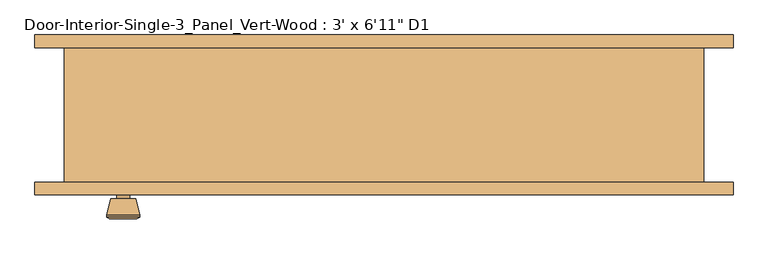
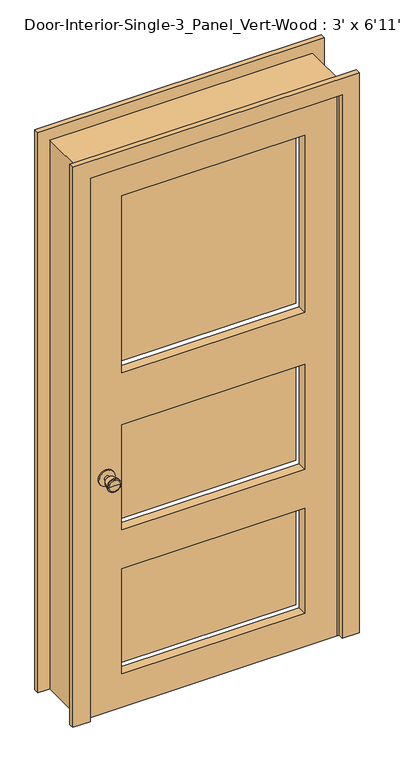
"""IFC4 building model written with IfcOpenShell, lengths in millimetres: door geometry."""

from ifc_helpers import new_model, si_unit, point, frame, frame_2d, origin, place, context, project, spatial, polyline, circle_curve, trimmed, segment, composite_curve, outline, extrude, faceted_brep, source, transform, mapped, element, save
from ifc_brep_helpers import plane_surface, cylinder_surface, revolved_surface, advanced_brep


def door_ac5ca1ae(model_context):
    return source(origin(), model_context, "Body", "SolidModel", [
        advanced_brep(
        [(-393.7, -57.5, 914.4), (-403.7, -57.5, 914.4), (-383.7, -57.5, 914.4), (-373.2241324, -8.5, 914.4), (-414.1758676, -8.5, 914.4), (-393.7, -8.5, 914.4), (-368.7, -10.3278681, 914.4), (-418.7, -10.3278681, 914.4), (-368.7, -13.7915463, 914.4), (-418.7, -13.7915463, 914.4), (-375.063764, -38.5, 914.4), (-412.336236, -38.5, 914.4), (-383.7, -38.5, 914.4), (-403.7, -38.5, 914.4)],
        [
            (0, 1),
            (1, 2, circle_curve(frame((-393.7, -57.5, 914.4), z_axis=(0.0, -1.0, 0.0), x_axis=(-1.0, 0.0, 0.0)), 10.0)),
            (2, 0),
            (2, 1, circle_curve(frame((-393.7, -57.5, 914.4), z_axis=(0.0, -1.0, 0.0), x_axis=(-1.0, 0.0, 0.0)), 10.0)),
            (3, 4, circle_curve(frame((-393.7, -8.5, 914.4), z_axis=(0.0, 1.0, 0.0), x_axis=(-1.0, 0.0, 0.0)), 20.4758676)),
            (4, 5),
            (5, 3),
            (4, 3, circle_curve(frame((-393.7, -8.5, 914.4), z_axis=(0.0, 1.0, 0.0), x_axis=(-1.0, 0.0, 0.0)), 20.4758676)),
            (6, 7, circle_curve(frame((-393.7, -10.3278681, 914.4), z_axis=(0.0, 1.0, 0.0), x_axis=(-1.0, 0.0, 0.0)), 25.0)),
            (7, 4),
            (3, 6),
            (7, 6, circle_curve(frame((-393.7, -10.3278681, 914.4), z_axis=(0.0, 1.0, 0.0), x_axis=(-1.0, 0.0, 0.0)), 25.0)),
            (8, 9, circle_curve(frame((-393.7, -13.7915463, 914.4), z_axis=(0.0, 1.0, 0.0), x_axis=(-1.0, 0.0, 0.0)), 25.0)),
            (9, 7),
            (6, 8),
            (9, 8, circle_curve(frame((-393.7, -13.7915463, 914.4), z_axis=(0.0, 1.0, 0.0), x_axis=(-1.0, 0.0, 0.0)), 25.0)),
            (10, 11, circle_curve(frame((-393.7, -38.5, 914.4), z_axis=(0.0, 1.0, 0.0), x_axis=(-1.0, 0.0, 0.0)), 18.636236)),
            (11, 9),
            (8, 10),
            (11, 10, circle_curve(frame((-393.7, -38.5, 914.4), z_axis=(0.0, 1.0, 0.0), x_axis=(-1.0, 0.0, 0.0)), 18.636236)),
            (12, 13, circle_curve(frame((-393.7, -38.5, 914.4), z_axis=(0.0, 1.0, 0.0), x_axis=(-1.0, 0.0, 0.0)), 10.0)),
            (13, 11),
            (10, 12),
            (13, 12, circle_curve(frame((-393.7, -38.5, 914.4), z_axis=(0.0, 1.0, 0.0), x_axis=(-1.0, 0.0, 0.0)), 10.0)),
            (1, 13),
            (12, 2),
        ],
        [
            plane_surface(frame((-393.7, -57.5, 914.4), z_axis=(0.0, -1.0, 0.0), x_axis=(-1.0, 0.0, 0.0))),
            plane_surface(frame((-393.7, -8.5, 914.4), z_axis=(0.0, 1.0, 0.0), x_axis=(-1.0, 0.0, 0.0))),
            revolved_surface(polyline([(-414.1758676, -8.5, 914.4), (-418.7, -10.3278681, 914.4)]), (-393.7, -57.5, 914.4), (0.0, -1.0, 0.0)),
            cylinder_surface(frame((-393.7, -57.5, 914.4), z_axis=(0.0, -1.0, 0.0), x_axis=(-1.0, 0.0, 0.0)), 25.0),
            revolved_surface(polyline([(-418.7, -13.7915463, 914.4), (-412.336236, -38.5, 914.4)]), (-393.7, -57.5, 914.4), (0.0, -1.0, 0.0)),
            plane_surface(frame((-393.7, -38.5, 914.4), z_axis=(0.0, -1.0, 0.0), x_axis=(-1.0, 0.0, 0.0))),
            cylinder_surface(frame((-393.7, -57.5, 914.4), z_axis=(0.0, -1.0, 0.0), x_axis=(-1.0, 0.0, 0.0)), 10.0),
        ],
        [
            (0, [[1, 2, 3]]),
            (0, [[-3, 4, -1]]),
            (1, [[5, 6, 7]]),
            (1, [[8, -7, -6]]),
            (2, [[9, 10, -5, 11]]),
            (2, [[12, -11, -8, -10]]),
            (3, [[13, 14, -9, 15]]),
            (3, [[16, -15, -12, -14]]),
            (4, [[17, 18, -13, 19]]),
            (4, [[20, -19, -16, -18]]),
            (5, [[21, 22, -17, 23]]),
            (5, [[24, -23, -20, -22]]),
            (6, [[-2, 25, -21, 26]]),
            (6, [[-4, -26, -24, -25]]),
        ],
    ),
        extrude(outline(composite_curve([segment(trimmed(circle_curve(frame_2d((914.4, -393.7)), 30.0), [point((914.4, -423.7))], [point((914.4, -363.7))], False, "CARTESIAN"), True, "CONTINUOUS"), segment(trimmed(circle_curve(frame_2d((914.4, -393.7)), 30.0), [point((914.4, -363.7))], [point((914.4, -423.7))], False, "CARTESIAN"), True, "CONTINUOUS")], self_intersect=False)), frame((0.0, -63.5, 0.0), z_axis=(0.0, 1.0, 0.0), x_axis=(0.0, 0.0, 1.0)), (0.0, 0.0, 1.0), 6.0),
        advanced_brep(
        [(-393.7, -104.425, 914.4), (-383.7, -104.425, 914.4), (-403.7, -104.425, 914.4), (-373.2241324, -153.425, 914.4), (-393.7, -153.425, 914.4), (-414.1758676, -153.425, 914.4), (-368.7, -151.5971319, 914.4), (-418.7, -151.5971319, 914.4), (-368.7, -148.1334537, 914.4), (-418.7, -148.1334537, 914.4), (-375.063764, -123.425, 914.4), (-412.336236, -123.425, 914.4), (-383.7, -123.425, 914.4), (-403.7, -123.425, 914.4)],
        [
            (0, 1),
            (1, 2, circle_curve(frame((-393.7, -104.425, 914.4), z_axis=(0.0, 1.0, 0.0), x_axis=(-1.0, 0.0, 0.0)), 10.0)),
            (2, 0),
            (2, 1, circle_curve(frame((-393.7, -104.425, 914.4), z_axis=(0.0, 1.0, 0.0), x_axis=(-1.0, 0.0, 0.0)), 10.0)),
            (3, 4),
            (4, 5),
            (5, 3, circle_curve(frame((-393.7, -153.425, 914.4), z_axis=(0.0, -1.0, 0.0), x_axis=(-1.0, 0.0, 0.0)), 20.4758676)),
            (3, 5, circle_curve(frame((-393.7, -153.425, 914.4), z_axis=(0.0, -1.0, 0.0), x_axis=(-1.0, 0.0, 0.0)), 20.4758676)),
            (6, 3),
            (5, 7),
            (7, 6, circle_curve(frame((-393.7, -151.5971319, 914.4), z_axis=(0.0, -1.0, 0.0), x_axis=(-1.0, 0.0, 0.0)), 25.0)),
            (6, 7, circle_curve(frame((-393.7, -151.5971319, 914.4), z_axis=(0.0, -1.0, 0.0), x_axis=(-1.0, 0.0, 0.0)), 25.0)),
            (8, 6),
            (7, 9),
            (9, 8, circle_curve(frame((-393.7, -148.1334537, 914.4), z_axis=(0.0, -1.0, 0.0), x_axis=(-1.0, 0.0, 0.0)), 25.0)),
            (8, 9, circle_curve(frame((-393.7, -148.1334537, 914.4), z_axis=(0.0, -1.0, 0.0), x_axis=(-1.0, 0.0, 0.0)), 25.0)),
            (10, 8),
            (9, 11),
            (11, 10, circle_curve(frame((-393.7, -123.425, 914.4), z_axis=(0.0, -1.0, 0.0), x_axis=(-1.0, 0.0, 0.0)), 18.636236)),
            (10, 11, circle_curve(frame((-393.7, -123.425, 914.4), z_axis=(0.0, -1.0, 0.0), x_axis=(-1.0, 0.0, 0.0)), 18.636236)),
            (12, 10),
            (11, 13),
            (13, 12, circle_curve(frame((-393.7, -123.425, 914.4), z_axis=(0.0, -1.0, 0.0), x_axis=(-1.0, 0.0, 0.0)), 10.0)),
            (12, 13, circle_curve(frame((-393.7, -123.425, 914.4), z_axis=(0.0, -1.0, 0.0), x_axis=(-1.0, 0.0, 0.0)), 10.0)),
            (1, 12),
            (13, 2),
        ],
        [
            plane_surface(frame((-393.7, -104.425, 914.4), z_axis=(0.0, 1.0, 0.0), x_axis=(-1.0, 0.0, 0.0))),
            plane_surface(frame((-393.7, -153.425, 914.4), z_axis=(0.0, -1.0, 0.0), x_axis=(-1.0, 0.0, 0.0))),
            revolved_surface(polyline([(-414.1758676, -153.425, 914.4), (-418.7, -151.5971319, 914.4)]), (-393.7, -104.425, 914.4), (0.0, 1.0, 0.0)),
            cylinder_surface(frame((-393.7, -104.425, 914.4), z_axis=(0.0, 1.0, 0.0), x_axis=(-1.0, 0.0, 0.0)), 25.0),
            revolved_surface(polyline([(-418.7, -148.1334537, 914.4), (-412.336236, -123.425, 914.4)]), (-393.7, -104.425, 914.4), (0.0, 1.0, 0.0)),
            plane_surface(frame((-393.7, -123.425, 914.4), z_axis=(0.0, 1.0, 0.0), x_axis=(-1.0, 0.0, 0.0))),
            cylinder_surface(frame((-393.7, -104.425, 914.4), z_axis=(0.0, 1.0, 0.0), x_axis=(-1.0, 0.0, 0.0)), 10.0),
        ],
        [
            (0, [[1, 2, 3]]),
            (0, [[-3, 4, -1]]),
            (1, [[5, 6, 7]]),
            (1, [[-6, -5, 8]]),
            (2, [[9, -7, 10, 11]]),
            (2, [[-10, -8, -9, 12]]),
            (3, [[13, -11, 14, 15]]),
            (3, [[-14, -12, -13, 16]]),
            (4, [[17, -15, 18, 19]]),
            (4, [[-18, -16, -17, 20]]),
            (5, [[21, -19, 22, 23]]),
            (5, [[-22, -20, -21, 24]]),
            (6, [[25, -23, 26, -2]]),
            (6, [[-26, -24, -25, -4]]),
        ],
    ),
        extrude(outline(composite_curve([segment(trimmed(circle_curve(frame_2d((914.4, -393.7)), 30.0), [point((914.4, -423.7))], [point((914.4, -363.7))], False, "CARTESIAN"), True, "CONTINUOUS"), segment(trimmed(circle_curve(frame_2d((914.4, -393.7)), 30.0), [point((914.4, -363.7))], [point((914.4, -423.7))], False, "CARTESIAN"), True, "CONTINUOUS")], self_intersect=False)), frame((0.0, -104.425, 0.0), z_axis=(0.0, 1.0, 0.0), x_axis=(0.0, 0.0, 1.0)), (0.0, 0.0, 1.0), 6.0),
        faceted_brep([(482.6, -98.425, 0.0), (457.2, -98.425, 0.0), (457.2, -63.5, 0.0), (444.5, -63.5, 0.0), (444.5, -28.575, 0.0), (457.2, -28.575, 0.0), (457.2, 104.775, 0.0), (482.6, 104.775, 0.0), (482.6, 104.775, 2133.6), (482.6, -98.425, 2133.6), (457.2, 104.775, 2108.2), (-457.2, 104.775, 2108.2), (-457.2, 104.775, 0.0), (-482.6, 104.775, 0.0), (-482.6, 104.775, 2133.6), (457.2, -28.575, 2108.2), (444.5, -28.575, 2095.5), (-444.5, -28.575, 2095.5), (-444.5, -28.575, 0.0), (-457.2, -28.575, 0.0), (-457.2, -28.575, 2108.2), (444.5, -63.5, 2095.5), (457.2, -63.5, 2108.2), (-457.2, -63.5, 2108.2), (-457.2, -63.5, 0.0), (-444.5, -63.5, 0.0), (-444.5, -63.5, 2095.5), (457.2, -98.425, 2108.2), (-482.6, -98.425, 2133.6), (-482.6, -98.425, 0.0), (-457.2, -98.425, 0.0), (-457.2, -98.425, 2108.2)], [[[0, 1, 2, 3, 4, 5, 6, 7]], [[7, 8, 9, 0]], [[6, 10, 11, 12, 13, 14, 8, 7]], [[5, 15, 10, 6]], [[4, 16, 17, 18, 19, 20, 15, 5]], [[3, 21, 16, 4]], [[2, 22, 23, 24, 25, 26, 21, 3]], [[1, 27, 22, 2]], [[0, 9, 28, 29, 30, 31, 27, 1]], [[8, 14, 28, 9]], [[15, 20, 11, 10]], [[21, 26, 17, 16]], [[27, 31, 23, 22]], [[29, 13, 12, 19, 18, 25, 24, 30]], [[14, 13, 29, 28]], [[20, 19, 12, 11]], [[26, 25, 18, 17]], [[31, 30, 24, 23]]]),
        extrude(outline(polyline([(2108.2, -457.2), (0.0, -457.2), (0.0, 457.2), (2108.2, 457.2), (2108.2, -457.2)]), holes=[polyline([(1989.1375, -336.55), (1989.1375, 336.55), (1301.75, 336.55), (1301.75, -336.55), (1989.1375, -336.55)]), polyline([(538.1625, -336.55), (538.1625, 336.55), (130.175, 336.55), (130.175, -336.55), (538.1625, -336.55)]), polyline([(1098.55, -336.55), (1098.55, 336.55), (690.5625, 336.55), (690.5625, -336.55), (1098.55, -336.55)])]), frame((0.0, -98.425, 0.0), z_axis=(0.0, 1.0, 0.0), x_axis=(0.0, 0.0, 1.0)), (0.0, 0.0, 1.0), 34.925),
        extrude(outline(polyline([(336.55, -30.6916667), (336.55, -42.3333333), (-336.55, -42.3333333), (-336.55, -30.6916667), (336.55, -30.6916667)])), frame((0.0, 0.0, 1301.75), z_axis=(0.0, 0.0, 1.0), x_axis=(1.0, 0.0, 0.0)), (0.0, 0.0, 1.0), 687.3875),
        extrude(outline(polyline([(336.55, -30.6916667), (336.55, -42.3333333), (-336.55, -42.3333333), (-336.55, -30.6916667), (336.55, -30.6916667)])), frame((0.0, 0.0, 130.175), z_axis=(0.0, 0.0, 1.0), x_axis=(1.0, 0.0, 0.0)), (0.0, 0.0, 1.0), 407.9875),
        extrude(outline(polyline([(336.55, -30.6916667), (336.55, -42.3333333), (-336.55, -42.3333333), (-336.55, -30.6916667), (336.55, -30.6916667)])), frame((0.0, 0.0, 690.5625), z_axis=(0.0, 0.0, 1.0), x_axis=(1.0, 0.0, 0.0)), (0.0, 0.0, 1.0), 407.9875),
        extrude(outline(polyline([(0.0, 527.05), (2178.05, 527.05), (2178.05, -527.05), (0.0, -527.05), (0.0, -463.55), (2114.55, -463.55), (2114.55, 463.55), (0.0, 463.55), (0.0, 527.05)])), frame((0.0, -117.475, 0.0), z_axis=(0.0, 1.0, 0.0), x_axis=(0.0, 0.0, 1.0)), (0.0, 0.0, 1.0), 19.05),
        extrude(outline(polyline([(0.0, 527.05), (2178.05, 527.05), (2178.05, -527.05), (0.0, -527.05), (0.0, -463.55), (2114.55, -463.55), (2114.55, 463.55), (0.0, 463.55), (0.0, 527.05)])), frame((0.0, 104.775, 0.0), z_axis=(0.0, 1.0, 0.0), x_axis=(0.0, 0.0, 1.0)), (0.0, 0.0, 1.0), 19.05),
    ])


if __name__ == "__main__":
    model = new_model("IFC4")
    model_context = context("Model", 3, world=origin())
    ifc_project = project(units=[si_unit("LENGTHUNIT", "METRE", prefix="MILLI")], contexts=[model_context])
    site = spatial("IfcSite", under=ifc_project)
    building = spatial("IfcBuilding", under=site)
    placement = place(None, origin())
    door_shape = door_ac5ca1ae(model_context)
    element("IfcDoor", 1, ObjectType="Door-Interior-Single-3_Panel_Vert-Wood : 3' x 6'11\" D1", at=placement, inside=building, context=model_context, shape_type="MappedRepresentation", body=[
        mapped(door_shape, transform((0.0, 0.0, 0.0), x_axis=(1.0, 0.0, 0.0), y_axis=(0.0, 1.0, 0.0), z_axis=(0.0, 0.0, 1.0))),
    ])
    save(model, "model.ifc")

# Revit data of these elements
# Type "Door-Interior-Single-3_Panel_Vert-Wood : 3' x 6'11\" D1"
#   Type Mark = "9"
#   Analytic Construction = "Wooden"
#   Top Rail = 0' - 4 11/16"
#   Thickness = 0' - 1 3/8"
#   Thermal Resistance (R) = 2.5876 (h·ft²·°F)/BTU
#   Swing Angle [instance default] = 90.00°
#   Stiles = 0' - 4 3/4"
#   Rough Width = 3' - 2"
#   Rough Height = 7' - 0"
#   Intermediate Rail = 0' - 4 1/2"
#   Height = 6' - 11"
#   Width = 3' - 0"
#   Heat Transfer Coefficient (U) = 0.3865 BTU/(h·ft²·°F)
#   Bottom Rail = 0' - 9 1/8"
#   Define Thermal Properties by = 1
#   Trim Material = Cherry
#   Panel Material = Cherry
#   Frame Material = Cherry
#   Door Handle Material = Aluminum
#   Visual Light Transmittance = 0
#   Solar Heat Gain Coefficient = 0
#   Wall Closure = (empty or 0)
#   Function = (empty or 0)
# Element 1 (IfcDoor, "Door-Interior-Single-3_Panel_Vert-Wood : 3' x 6'11\" D1")
#   Materials on its faces: "Cherry", "Aluminum"
# Materials
#   "Cherry": class "Wood", colour RGB 226 177 128, transparency 0, Description = "Prunus Serotina", Cost = 0
#   "Aluminum": class "Metal", colour RGB 247 247 247, transparency 0, Description = "Aluminum 6061", Cost = 0
